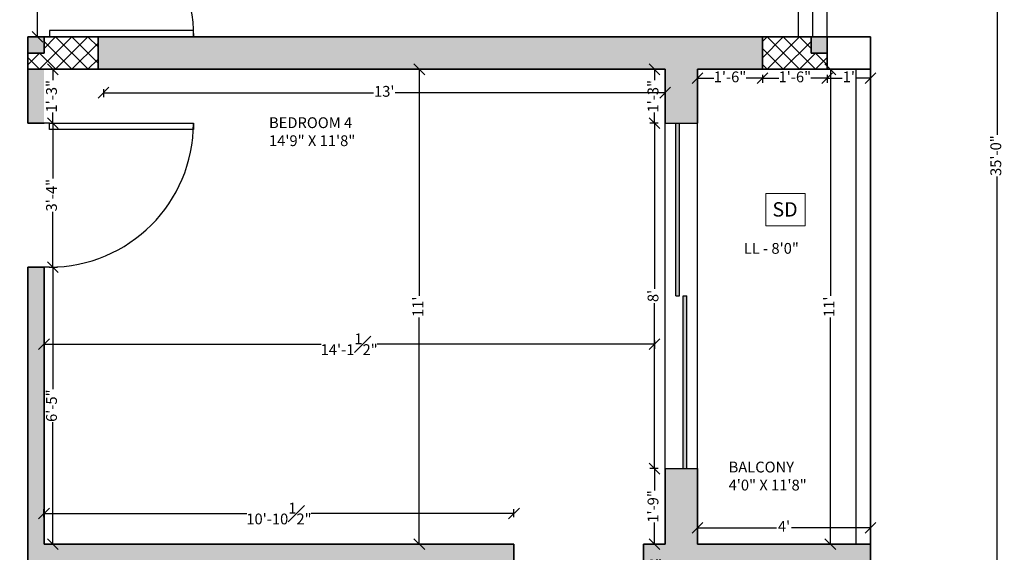
# Model space of a CAD drawing. Units: inches. Extents: x 1365 to 2091, y 1589 to 2091.
# Tile 7 of 8: x 1818 to 2091, y 1743 to 1891. Entities that reach past the tile are written whole.
import ezdxf

# ---------------------------------------------------------------- set-up
doc = ezdxf.new("R2010")
doc.units = ezdxf.units.IN
for name, color, linetype, lineweight in [('A-ANNO-DIMS', 2, 'Continuous', 18), ('A-ANNO-SYMB', 12, 'Continuous', 18), ('A-AREA-IDEN', 7, 'Continuous', 18), ('A-COLS', 7, 'Continuous', 35), ('A-COLS-MARK-PATT', 114, 'Continuous', 13), ('A-COLS-PATT', 1, 'Continuous', 13), ('A-DOOR', 4, 'Continuous', 25), ('A-DOOR-PATT', 143, 'Continuous', 13), ('A-FLOR-HRAL', 7, 'Continuous', 25), ('A-WALL', 7, 'Continuous', 35), ('A-WALL-PATT', 253, 'Continuous', 13)]:
    doc.layers.add(name, color=color, linetype=linetype, lineweight=lineweight)
doc.styles.get("Standard").update_dxf_attribs({"font": 'arial.ttf'})
doc.dimstyles.new('ISO-25', dxfattribs={"dimtxt": 3, "dimasz": 3, "dimexe": 1.25, "dimexo": 0.625, "dimtad": 0, "dimlunit": 4, "dimtxsty": 'Standard', "dimblk": 'OBLIQUE', "dimcen": 2.5, "dimclrd": 254, "dimclre": 254, "dimclrt": 1, "dimadec": 0, "dimazin": 0, "dimtfac": 1, "dimtmove": 0, "dimatfit": 3, "dimfxl": 1, "dimfxlon": 1, "dimfrac": 1, "dimarcsym": 0})

# ---------------------------------------------------------------- blocks, each defined once
blk = doc.blocks.new('*U5')
for p, q in [((0, 0), (0, -6)), ((40, 0), (40, -6))]:
    blk.add_line(p, q)
blk.add_lwpolyline([(0, 0), (0, 40), (1.75, 40), (1.75, 0)], close=True)
blk.add_arc((0, 0), 40, 0, 90)
blk = doc.blocks.new('_Oblique')
at = {"color": 0, "linetype": 'ByBlock', "lineweight": -2}
blk.add_line((-0.5, -0.5), (0.5, 0.5), dxfattribs=at)
blk = doc.blocks.new('*D61')
at = {"layer": 'A-ANNO-DIMS', "color": 0, "lineweight": -2, "transparency": 16777216}
for p, q in [((1929.47, 1876.86), (1927.22, 1876.86)), ((1928.47, 1876.86), (1928.47, 1813.89)), ((1928.47, 1744.86), (1928.47, 1807.83)), ((1929.47, 1744.86), (1927.22, 1744.86))]:
    blk.add_line(p, q, dxfattribs=at)
at = {"layer": 'Defpoints', "color": 0, "transparency": 16777216}
for p in [(1939.4, 1876.86), (1928.47, 1744.86), (1939.4, 1744.86)]:
    blk.add_point(p, dxfattribs=at)
at = {"layer": 'A-ANNO-DIMS', "color": 0, "lineweight": -2, "transparency": 16777216, "xscale": 3, "yscale": 3, "zscale": 3}
for p, rotation in [((1928.47, 1876.86), 90), ((1928.47, 1744.86), 270)]:
    blk.add_blockref('_Oblique', p, dxfattribs=dict(at, rotation=rotation))
at = {"layer": 'A-ANNO-DIMS', "color": 0, "transparency": 16777216, "insert": (1928.47, 1810.86), "char_height": 3, "attachment_point": 5, "rotation": 90}
blk.add_mtext("11'", dxfattribs=at)
blk = doc.blocks.new('*D62')
at = {"layer": 'A-ANNO-DIMS', "color": 0, "lineweight": -2, "transparency": 16777216}
for p, q in [((1825.72, 1876.86), (1827.97, 1876.86)), ((1826.72, 1876.86), (1826.72, 1873.83)), ((1826.72, 1861.86), (1826.72, 1864.89)), ((1825.72, 1861.86), (1827.97, 1861.86))]:
    blk.add_line(p, q, dxfattribs=at)
at = {"layer": 'Defpoints', "color": 0, "transparency": 16777216}
for p in [(1824.34, 1876.86), (1824.25, 1861.86), (1826.72, 1861.86)]:
    blk.add_point(p, dxfattribs=at)
at = {"layer": 'A-ANNO-DIMS', "color": 0, "lineweight": -2, "transparency": 16777216, "xscale": 3, "yscale": 3, "zscale": 3}
for p, rotation in [((1826.72, 1876.86), 90), ((1826.72, 1861.86), 270)]:
    blk.add_blockref('_Oblique', p, dxfattribs=dict(at, rotation=rotation))
at = {"layer": 'A-ANNO-DIMS', "color": 0, "transparency": 16777216, "insert": (1826.72, 1869.36), "char_height": 3, "attachment_point": 5, "rotation": 90}
blk.add_mtext('1\'-3"', dxfattribs=at)
blk = doc.blocks.new('*D63')
at = {"layer": 'A-ANNO-DIMS', "color": 0, "lineweight": -2, "transparency": 16777216}
for p, q in [((1825.72, 1861.86), (1827.97, 1861.86)), ((1826.72, 1861.86), (1826.72, 1846.47)), ((1826.72, 1821.86), (1826.72, 1837.25)), ((1825.72, 1821.86), (1827.97, 1821.86))]:
    blk.add_line(p, q, dxfattribs=at)
at = {"layer": 'Defpoints', "color": 0, "transparency": 16777216}
for p in [(1824.25, 1861.86), (1819.75, 1821.86), (1826.72, 1821.86)]:
    blk.add_point(p, dxfattribs=at)
at = {"layer": 'A-ANNO-DIMS', "color": 0, "lineweight": -2, "transparency": 16777216, "xscale": 3, "yscale": 3, "zscale": 3}
for p, rotation in [((1826.72, 1861.86), 90), ((1826.72, 1821.86), 270)]:
    blk.add_blockref('_Oblique', p, dxfattribs=dict(at, rotation=rotation))
at = {"layer": 'A-ANNO-DIMS', "color": 0, "transparency": 16777216, "insert": (1826.72, 1841.86), "char_height": 3, "attachment_point": 5, "rotation": 90}
blk.add_mtext('3\'-4"', dxfattribs=at)
blk = doc.blocks.new('*D64')
at = {"layer": 'A-ANNO-DIMS', "color": 0, "lineweight": -2, "transparency": 16777216}
for p, q in [((1825.72, 1821.86), (1827.97, 1821.86)), ((1826.72, 1821.86), (1826.72, 1787.98)), ((1826.72, 1744.86), (1826.72, 1778.74)), ((1825.72, 1744.86), (1827.97, 1744.86))]:
    blk.add_line(p, q, dxfattribs=at)
at = {"layer": 'Defpoints', "color": 0, "transparency": 16777216}
for p in [(1819.75, 1821.86), (1824.25, 1744.86), (1826.72, 1744.86)]:
    blk.add_point(p, dxfattribs=at)
at = {"layer": 'A-ANNO-DIMS', "color": 0, "lineweight": -2, "transparency": 16777216, "xscale": 3, "yscale": 3, "zscale": 3}
for p, rotation in [((1826.72, 1821.86), 90), ((1826.72, 1744.86), 270)]:
    blk.add_blockref('_Oblique', p, dxfattribs=dict(at, rotation=rotation))
at = {"layer": 'A-ANNO-DIMS', "color": 0, "transparency": 16777216, "insert": (1826.72, 1783.36), "char_height": 3, "attachment_point": 5, "rotation": 90}
blk.add_mtext('6\'-5"', dxfattribs=at)
blk = doc.blocks.new('*D65')
at = {"layer": 'A-ANNO-DIMS', "color": 0, "lineweight": -2, "transparency": 16777216}
for p, q in [((1824.25, 1752.38), (1824.25, 1754.63)), ((1824.25, 1753.38), (1880.56, 1753.38)), ((1954.75, 1753.38), (1898.45, 1753.38)), ((1954.75, 1752.38), (1954.75, 1754.63))]:
    blk.add_line(p, q, dxfattribs=at)
at = {"layer": 'Defpoints', "color": 0, "transparency": 16777216}
for p in [(1954.75, 1753.38), (1824.25, 1744.86), (1954.75, 1744.86)]:
    blk.add_point(p, dxfattribs=at)
at = {"layer": 'A-ANNO-DIMS', "color": 0, "lineweight": -2, "transparency": 16777216, "xscale": 3, "yscale": 3, "zscale": 3, "rotation": 180}
blk.add_blockref('_Oblique', (1824.25, 1753.38), dxfattribs=at)
at = {"layer": 'A-ANNO-DIMS', "color": 0, "lineweight": -2, "transparency": 16777216, "xscale": 3, "yscale": 3, "zscale": 3}
blk.add_blockref('_Oblique', (1954.75, 1753.38), dxfattribs=at)
at = {"layer": 'A-ANNO-DIMS', "color": 0, "transparency": 16777216, "insert": (1889.5, 1753.38), "char_height": 3, "attachment_point": 5}
blk.add_mtext('10\'-10{\\H1x;\\S1#2;}"', dxfattribs=at)
blk = doc.blocks.new('*D66')
at = {"layer": 'A-ANNO-DIMS', "color": 0, "lineweight": -2, "transparency": 16777216}
for p, q in [((1840.75, 1871.34), (1840.75, 1869.09)), ((1840.75, 1870.34), (1915.72, 1870.34)), ((1996.75, 1870.34), (1921.78, 1870.34)), ((1996.75, 1871.34), (1996.75, 1869.09))]:
    blk.add_line(p, q, dxfattribs=at)
at = {"layer": 'Defpoints', "color": 0, "transparency": 16777216}
for p in [(1840.75, 1876.86), (1996.75, 1876.86), (1840.75, 1870.34)]:
    blk.add_point(p, dxfattribs=at)
at = {"layer": 'A-ANNO-DIMS', "color": 0, "lineweight": -2, "transparency": 16777216, "xscale": 3, "yscale": 3, "zscale": 3, "rotation": 180}
blk.add_blockref('_Oblique', (1840.75, 1870.34), dxfattribs=at)
at = {"layer": 'A-ANNO-DIMS', "color": 0, "lineweight": -2, "transparency": 16777216, "xscale": 3, "yscale": 3, "zscale": 3}
blk.add_blockref('_Oblique', (1996.75, 1870.34), dxfattribs=at)
at = {"layer": 'A-ANNO-DIMS', "color": 0, "transparency": 16777216, "insert": (1918.75, 1870.34), "char_height": 3, "attachment_point": 5}
blk.add_mtext("13'", dxfattribs=at)
blk = doc.blocks.new('*D67')
at = {"layer": 'A-ANNO-DIMS', "color": 0, "lineweight": -2, "transparency": 16777216}
for p, q in [((1994.76, 1765.86), (1992.51, 1765.86)), ((1993.76, 1765.86), (1993.76, 1759.83)), ((1993.76, 1744.86), (1993.76, 1750.89)), ((1994.76, 1744.86), (1992.51, 1744.86))]:
    blk.add_line(p, q, dxfattribs=at)
at = {"layer": 'Defpoints', "color": 0, "transparency": 16777216}
for p in [(1993.76, 1765.86), (1996.75, 1765.86), (1996.75, 1744.86)]:
    blk.add_point(p, dxfattribs=at)
at = {"layer": 'A-ANNO-DIMS', "color": 0, "lineweight": -2, "transparency": 16777216, "xscale": 3, "yscale": 3, "zscale": 3}
for p, rotation in [((1993.76, 1765.86), 90), ((1993.76, 1744.86), 270)]:
    blk.add_blockref('_Oblique', p, dxfattribs=dict(at, rotation=rotation))
at = {"layer": 'A-ANNO-DIMS', "color": 0, "transparency": 16777216, "insert": (1993.76, 1755.36), "char_height": 3, "attachment_point": 5, "rotation": 90}
blk.add_mtext('1\'-9"', dxfattribs=at)
blk = doc.blocks.new('*D68')
at = {"layer": 'A-ANNO-DIMS', "color": 0, "lineweight": -2, "transparency": 16777216}
for p, q in [((1990.75, 1739.68), (1990.75, 1737.43)), ((1996.75, 1739.68), (1996.75, 1737.43)), ((1990.75, 1738.68), (1991.4, 1738.68)), ((1996.75, 1738.68), (1996.11, 1738.68))]:
    blk.add_line(p, q, dxfattribs=at)
at = {"layer": 'Defpoints', "color": 0, "transparency": 16777216}
for p in [(1990.75, 1744.86), (1996.75, 1744.86), (1996.75, 1738.68)]:
    blk.add_point(p, dxfattribs=at)
at = {"layer": 'A-ANNO-DIMS', "color": 0, "lineweight": -2, "transparency": 16777216, "xscale": 3, "yscale": 3, "zscale": 3, "rotation": 180}
blk.add_blockref('_Oblique', (1990.75, 1738.68), dxfattribs=at)
at = {"layer": 'A-ANNO-DIMS', "color": 0, "lineweight": -2, "transparency": 16777216, "xscale": 3, "yscale": 3, "zscale": 3}
blk.add_blockref('_Oblique', (1996.75, 1738.68), dxfattribs=at)
at = {"layer": 'A-ANNO-DIMS', "color": 0, "transparency": 16777216, "insert": (1993.75, 1738.68), "char_height": 3, "attachment_point": 5}
blk.add_mtext('6"', dxfattribs=at)
blk = doc.blocks.new('*D69')
at = {"layer": 'A-ANNO-DIMS', "color": 0, "lineweight": -2, "transparency": 16777216}
for p, q in [((1994.76, 1861.86), (1992.51, 1861.86)), ((1993.76, 1861.86), (1993.76, 1815.86)), ((1993.76, 1765.86), (1993.76, 1811.85)), ((1994.76, 1765.86), (1992.51, 1765.86))]:
    blk.add_line(p, q, dxfattribs=at)
at = {"layer": 'Defpoints', "color": 0, "transparency": 16777216}
for p in [(1993.76, 1861.86), (1996.75, 1861.86), (1996.75, 1765.86)]:
    blk.add_point(p, dxfattribs=at)
at = {"layer": 'A-ANNO-DIMS', "color": 0, "lineweight": -2, "transparency": 16777216, "xscale": 3, "yscale": 3, "zscale": 3}
for p, rotation in [((1993.76, 1861.86), 90), ((1993.76, 1765.86), 270)]:
    blk.add_blockref('_Oblique', p, dxfattribs=dict(at, rotation=rotation))
at = {"layer": 'A-ANNO-DIMS', "color": 0, "transparency": 16777216, "insert": (1993.76, 1813.86), "char_height": 3, "attachment_point": 5, "rotation": 90}
blk.add_mtext("8'", dxfattribs=at)
blk = doc.blocks.new('*D70')
at = {"layer": 'A-ANNO-DIMS', "color": 0, "lineweight": -2, "transparency": 16777216}
for p, q in [((1994.76, 1876.86), (1992.51, 1876.86)), ((1993.76, 1876.86), (1993.76, 1873.83)), ((1993.76, 1861.86), (1993.76, 1864.89)), ((1994.76, 1861.86), (1992.51, 1861.86))]:
    blk.add_line(p, q, dxfattribs=at)
at = {"layer": 'Defpoints', "color": 0, "transparency": 16777216}
for p in [(1993.76, 1876.86), (1996.75, 1876.86), (1996.75, 1861.86)]:
    blk.add_point(p, dxfattribs=at)
at = {"layer": 'A-ANNO-DIMS', "color": 0, "lineweight": -2, "transparency": 16777216, "xscale": 3, "yscale": 3, "zscale": 3}
for p, rotation in [((1993.76, 1876.86), 90), ((1993.76, 1861.86), 270)]:
    blk.add_blockref('_Oblique', p, dxfattribs=dict(at, rotation=rotation))
at = {"layer": 'A-ANNO-DIMS', "color": 0, "transparency": 16777216, "insert": (1993.76, 1869.36), "char_height": 3, "attachment_point": 5, "rotation": 90}
blk.add_mtext('1\'-3"', dxfattribs=at)
blk = doc.blocks.new('*D71')
at = {"layer": 'A-ANNO-DIMS', "color": 0, "lineweight": -2, "transparency": 16777216}
for p, q in [((2005.75, 1875.36), (2005.75, 1873.11)), ((2005.75, 1874.36), (2010.28, 1874.36)), ((2023.75, 1874.36), (2019.22, 1874.36)), ((2023.75, 1875.36), (2023.75, 1873.11))]:
    blk.add_line(p, q, dxfattribs=at)
at = {"layer": 'Defpoints', "color": 0, "transparency": 16777216}
for p in [(2005.75, 1876.86), (2023.75, 1876.86), (2023.75, 1874.36)]:
    blk.add_point(p, dxfattribs=at)
at = {"layer": 'A-ANNO-DIMS', "color": 0, "lineweight": -2, "transparency": 16777216, "xscale": 3, "yscale": 3, "zscale": 3, "rotation": 180}
blk.add_blockref('_Oblique', (2005.75, 1874.36), dxfattribs=at)
at = {"layer": 'A-ANNO-DIMS', "color": 0, "lineweight": -2, "transparency": 16777216, "xscale": 3, "yscale": 3, "zscale": 3}
blk.add_blockref('_Oblique', (2023.75, 1874.36), dxfattribs=at)
at = {"layer": 'A-ANNO-DIMS', "color": 0, "transparency": 16777216, "insert": (2014.75, 1874.36), "char_height": 3, "attachment_point": 5}
blk.add_mtext('1\'-6"', dxfattribs=at)
blk = doc.blocks.new('*D72')
at = {"layer": 'A-ANNO-DIMS', "color": 0, "lineweight": -2, "transparency": 16777216}
for p, q in [((2023.75, 1875.36), (2023.75, 1873.11)), ((2023.75, 1874.36), (2028.28, 1874.36)), ((2041.75, 1874.36), (2037.22, 1874.36)), ((2041.75, 1875.36), (2041.75, 1873.11))]:
    blk.add_line(p, q, dxfattribs=at)
at = {"layer": 'Defpoints', "color": 0, "transparency": 16777216}
for p in [(2023.75, 1876.86), (2041.75, 1876.86), (2041.75, 1874.36)]:
    blk.add_point(p, dxfattribs=at)
at = {"layer": 'A-ANNO-DIMS', "color": 0, "lineweight": -2, "transparency": 16777216, "xscale": 3, "yscale": 3, "zscale": 3, "rotation": 180}
blk.add_blockref('_Oblique', (2023.75, 1874.36), dxfattribs=at)
at = {"layer": 'A-ANNO-DIMS', "color": 0, "lineweight": -2, "transparency": 16777216, "xscale": 3, "yscale": 3, "zscale": 3}
blk.add_blockref('_Oblique', (2041.75, 1874.36), dxfattribs=at)
at = {"layer": 'A-ANNO-DIMS', "color": 0, "transparency": 16777216, "insert": (2032.75, 1874.36), "char_height": 3, "attachment_point": 5}
blk.add_mtext('1\'-6"', dxfattribs=at)
blk = doc.blocks.new('*D73')
at = {"layer": 'A-ANNO-DIMS', "color": 0, "lineweight": -2, "transparency": 16777216}
for p, q in [((2041.75, 1875.36), (2041.75, 1873.11)), ((2041.75, 1874.36), (2045.89, 1874.36)), ((2053.75, 1874.36), (2049.62, 1874.36)), ((2053.75, 1875.36), (2053.75, 1873.11))]:
    blk.add_line(p, q, dxfattribs=at)
at = {"layer": 'Defpoints', "color": 0, "transparency": 16777216}
for p in [(2041.75, 1876.86), (2053.75, 1876.86), (2053.75, 1874.36)]:
    blk.add_point(p, dxfattribs=at)
at = {"layer": 'A-ANNO-DIMS', "color": 0, "lineweight": -2, "transparency": 16777216, "xscale": 3, "yscale": 3, "zscale": 3, "rotation": 180}
blk.add_blockref('_Oblique', (2041.75, 1874.36), dxfattribs=at)
at = {"layer": 'A-ANNO-DIMS', "color": 0, "lineweight": -2, "transparency": 16777216, "xscale": 3, "yscale": 3, "zscale": 3}
blk.add_blockref('_Oblique', (2053.75, 1874.36), dxfattribs=at)
at = {"layer": 'A-ANNO-DIMS', "color": 0, "transparency": 16777216, "insert": (2047.75, 1874.36), "char_height": 3, "attachment_point": 5}
blk.add_mtext("1'", dxfattribs=at)
blk = doc.blocks.new('*D74')
at = {"layer": 'A-ANNO-DIMS', "color": 0, "lineweight": -2, "transparency": 16777216}
for p, q in [((2043.63, 1876.86), (2041.38, 1876.86)), ((2042.63, 1876.86), (2042.63, 1813.89)), ((2042.63, 1744.86), (2042.63, 1807.83)), ((2043.63, 1744.86), (2041.38, 1744.86))]:
    blk.add_line(p, q, dxfattribs=at)
at = {"layer": 'Defpoints', "color": 0, "transparency": 16777216}
for p in [(2053.75, 1876.86), (2042.63, 1744.86), (2053.75, 1744.86)]:
    blk.add_point(p, dxfattribs=at)
at = {"layer": 'A-ANNO-DIMS', "color": 0, "lineweight": -2, "transparency": 16777216, "xscale": 3, "yscale": 3, "zscale": 3}
for p, rotation in [((2042.63, 1876.86), 90), ((2042.63, 1744.86), 270)]:
    blk.add_blockref('_Oblique', p, dxfattribs=dict(at, rotation=rotation))
at = {"layer": 'A-ANNO-DIMS', "color": 0, "transparency": 16777216, "insert": (2042.63, 1810.86), "char_height": 3, "attachment_point": 5, "rotation": 90}
blk.add_mtext("11'", dxfattribs=at)
blk = doc.blocks.new('*D75')
at = {"layer": 'A-ANNO-DIMS', "color": 0, "lineweight": -2, "transparency": 16777216}
for p, q in [((2005.75, 1748.43), (2005.75, 1750.68)), ((2053.75, 1748.43), (2053.75, 1750.68)), ((2005.75, 1749.43), (2027.69, 1749.43)), ((2053.75, 1749.43), (2031.82, 1749.43))]:
    blk.add_line(p, q, dxfattribs=at)
at = {"layer": 'Defpoints', "color": 0, "transparency": 16777216}
for p in [(2053.75, 1749.43), (2005.75, 1744.86), (2053.75, 1744.86)]:
    blk.add_point(p, dxfattribs=at)
at = {"layer": 'A-ANNO-DIMS', "color": 0, "lineweight": -2, "transparency": 16777216, "xscale": 3, "yscale": 3, "zscale": 3, "rotation": 180}
blk.add_blockref('_Oblique', (2005.75, 1749.43), dxfattribs=at)
at = {"layer": 'A-ANNO-DIMS', "color": 0, "lineweight": -2, "transparency": 16777216, "xscale": 3, "yscale": 3, "zscale": 3}
blk.add_blockref('_Oblique', (2053.75, 1749.43), dxfattribs=at)
at = {"layer": 'A-ANNO-DIMS', "color": 0, "transparency": 16777216, "insert": (2029.75, 1749.43), "char_height": 3, "attachment_point": 5}
blk.add_mtext("4'", dxfattribs=at)
blk = doc.blocks.new('*D86')
at = {"layer": 'A-ANNO-DIMS', "color": 0, "lineweight": -2, "transparency": 16777216}
for p, q in [((1824.25, 1801.44), (1824.25, 1799.19)), ((1824.25, 1800.44), (1901.22, 1800.44)), ((1993.76, 1800.44), (1916.79, 1800.44)), ((1993.76, 1801.44), (1993.76, 1799.19))]:
    blk.add_line(p, q, dxfattribs=at)
at = {"layer": 'Defpoints', "color": 0, "transparency": 16777216}
for p in [(1824.25, 1821.86), (1993.76, 1821.86), (1993.76, 1800.44)]:
    blk.add_point(p, dxfattribs=at)
at = {"layer": 'A-ANNO-DIMS', "color": 0, "lineweight": -2, "transparency": 16777216, "xscale": 3, "yscale": 3, "zscale": 3, "rotation": 180}
blk.add_blockref('_Oblique', (1824.25, 1800.44), dxfattribs=at)
at = {"layer": 'A-ANNO-DIMS', "color": 0, "lineweight": -2, "transparency": 16777216, "xscale": 3, "yscale": 3, "zscale": 3}
blk.add_blockref('_Oblique', (1993.76, 1800.44), dxfattribs=at)
at = {"layer": 'A-ANNO-DIMS', "color": 0, "transparency": 16777216, "insert": (1909, 1800.44), "char_height": 3, "attachment_point": 5}
blk.add_mtext('14\'-1{\\H1x;\\S1#2;}"', dxfattribs=at)
blk = doc.blocks.new('*D92')
at = {"layer": 'A-ANNO-DIMS', "color": 0, "lineweight": -2, "transparency": 16777216}
for p, q in [((1821.45, 1925.83), (1823.7, 1925.83)), ((1822.45, 1925.83), (1822.45, 1910.45)), ((1822.45, 1885.86), (1822.45, 1901.23)), ((1821.45, 1885.86), (1823.7, 1885.86))]:
    blk.add_line(p, q, dxfattribs=at)
at = {"layer": 'Defpoints', "color": 0, "transparency": 16777216}
for p in [(1819.75, 1925.83), (1819.75, 1885.86), (1822.45, 1885.86)]:
    blk.add_point(p, dxfattribs=at)
at = {"layer": 'A-ANNO-DIMS', "color": 0, "lineweight": -2, "transparency": 16777216, "xscale": 3, "yscale": 3, "zscale": 3}
for p, rotation in [((1822.45, 1925.83), 90), ((1822.45, 1885.86), 270)]:
    blk.add_blockref('_Oblique', p, dxfattribs=dict(at, rotation=rotation))
at = {"layer": 'A-ANNO-DIMS', "color": 0, "transparency": 16777216, "insert": (1822.45, 1905.84), "char_height": 3, "attachment_point": 5, "rotation": 90}
blk.add_mtext('3\'-4"', dxfattribs=at)
blk = doc.blocks.new('*D123')
at = {"layer": 'A-ANNO-DIMS', "color": 254, "lineweight": -2, "transparency": 16777216}
for p, q in [((2087.95, 2062.86), (2090.2, 2062.86)), ((2088.95, 2062.86), (2088.95, 1858.63)), ((2088.95, 1642.86), (2088.95, 1847.08)), ((2087.95, 1642.86), (2090.2, 1642.86))]:
    blk.add_line(p, q, dxfattribs=at)
at = {"layer": 'Defpoints', "color": 0, "transparency": 16777216}
for p in [(2053.75, 2062.86), (2088.95, 2062.86), (2053.75, 1642.86)]:
    blk.add_point(p, dxfattribs=at)
at = {"layer": 'A-ANNO-DIMS', "color": 254, "lineweight": -2, "transparency": 16777216, "xscale": 3, "yscale": 3, "zscale": 3}
for p, rotation in [((2088.95, 2062.86), 90), ((2088.95, 1642.86), 270)]:
    blk.add_blockref('_Oblique', p, dxfattribs=dict(at, rotation=rotation))
at = {"layer": 'A-ANNO-DIMS', "color": 1, "transparency": 16777216, "insert": (2088.95, 1852.86), "char_height": 3, "attachment_point": 5, "rotation": 90}
blk.add_mtext('35\'-0"', dxfattribs=at)

msp = doc.modelspace()

# ---------------------------------------------------------------- hatches: boundary and pattern name
at = {"layer": 'A-COLS-MARK-PATT'}
h = msp.add_hatch(color=256, dxfattribs=at)
h.dxf.hatch_style = 1
h.paths.add_polyline_path([(1398.254, 2062.858), (1393.754, 2062.858), (1393.754, 2058.358), (1398.254, 2058.358)])
h.paths.add_polyline_path([(1398.254, 1872.358), (1393.754, 1872.358), (1393.754, 1867.858), (1398.254, 1867.858)])
h.paths.add_polyline_path([(1398.254, 1807.858), (1393.754, 1807.858), (1393.754, 1803.358), (1398.254, 1803.358)])
h.paths.add_polyline_path([(1398.254, 1647.358), (1393.754, 1647.358), (1393.754, 1642.858), (1398.254, 1642.858)])
h.paths.add_polyline_path([(1638.254, 1647.358), (1633.754, 1647.358), (1633.754, 1642.858), (1638.254, 1642.858)])
h.paths.add_polyline_path([(1638.254, 1732.858), (1633.754, 1732.858), (1633.754, 1728.358), (1638.254, 1728.358)])
h.paths.add_polyline_path([(1647.254, 1876.858), (1642.754, 1876.858), (1642.754, 1872.358), (1647.254, 1872.358)])
h.paths.add_polyline_path([(1647.254, 1803.358), (1642.754, 1803.358), (1642.754, 1798.858), (1647.254, 1798.858)])
h.paths.add_polyline_path([(1647.254, 2062.858), (1642.754, 2062.858), (1642.754, 2058.358), (1647.254, 2058.358)])
h.paths.add_polyline_path([(1824.254, 2062.858), (1819.754, 2062.858), (1819.754, 2058.358), (1824.254, 2058.358)])
h.paths.add_polyline_path([(1824.254, 1885.858), (1819.754, 1885.858), (1819.754, 1881.358), (1824.254, 1881.358)])
h.paths.add_polyline_path([(1828.754, 1647.358), (1824.254, 1647.358), (1824.254, 1642.858), (1828.754, 1642.858)])
h.paths.add_polyline_path([(1948.754, 1647.358), (1944.254, 1647.358), (1944.254, 1642.858), (1948.754, 1642.858)])
h.paths.add_polyline_path([(2041.754, 1647.358), (2037.254, 1647.358), (2037.254, 1642.858), (2041.754, 1642.858)])
h.paths.add_polyline_path([(2041.754, 1885.858), (2037.254, 1885.858), (2037.254, 1881.358), (2041.754, 1881.358)])
h.paths.add_polyline_path([(2041.754, 2062.858), (2037.254, 2062.858), (2037.254, 2058.358), (2041.754, 2058.358)])
at = {"layer": 'A-COLS-PATT'}
h = msp.add_hatch(dxfattribs=at)
h.set_pattern_fill('ANSI37', color=256)
h.paths.add_polyline_path([(1642.754, 1803.358), (1647.254, 1803.358), (1647.254, 1807.858), (1629.254, 1807.858), (1629.254, 1798.858), (1633.754, 1798.858), (1642.754, 1798.858)])
h.paths.add_polyline_path([(1647.254, 1872.358), (1642.754, 1872.358), (1642.754, 1876.858), (1641.254, 1876.858), (1623.254, 1876.858), (1623.254, 1867.858), (1638.254, 1867.858), (1647.254, 1867.858)])
h.paths.add_polyline_path([(1647.254, 2058.358), (1642.754, 2058.358), (1642.754, 2062.858), (1638.254, 2062.858), (1638.254, 2053.858), (1647.254, 2053.858)])
h.paths.add_polyline_path([(1642.754, 2053.858), (1638.254, 2053.858), (1638.254, 2041.858), (1642.754, 2041.858)])
h.paths.add_polyline_path([(1647.254, 2053.858), (1642.754, 2053.858), (1642.754, 2041.858), (1647.254, 2041.858)])
h.paths.add_polyline_path([(1828.754, 2062.858), (1824.254, 2062.858), (1824.254, 2058.358), (1819.754, 2058.358), (1819.754, 2038.858), (1828.754, 2038.858)])
h.paths.add_polyline_path([(1839.254, 1885.858), (1825.754, 1885.858), (1824.254, 1885.858), (1824.254, 1881.358), (1819.754, 1881.358), (1819.754, 1876.858), (1839.254, 1876.858)])
h.paths.add_polyline_path([(2041.754, 1881.358), (2037.254, 1881.358), (2037.254, 1885.858), (2023.754, 1885.858), (2023.754, 1876.858), (2041.754, 1876.858)])
h.paths.add_polyline_path([(1828.754, 1666.858), (1819.754, 1666.858), (1819.754, 1642.858), (1824.254, 1642.858), (1824.254, 1647.358), (1828.754, 1647.358)])
h.paths.add_polyline_path([(1944.254, 1647.358), (1948.754, 1647.358), (1948.754, 1651.858), (1930.754, 1651.858), (1930.754, 1642.858), (1944.254, 1642.858)])
h.paths.add_polyline_path([(2037.254, 1647.358), (2041.754, 1647.358), (2041.754, 1651.858), (2023.754, 1651.858), (2023.754, 1642.858), (2037.254, 1642.858)])
at = {"layer": 'A-DOOR-PATT'}
h = msp.add_hatch(color=256, dxfattribs=at)
h.dxf.hatch_style = 1
h.paths.add_polyline_path([(2000.754, 1861.858), (1999.754, 1861.858), (1999.754, 1813.858), (2000.754, 1813.858)])
h.paths.add_polyline_path([(2002.754, 1813.858), (2001.754, 1813.858), (2001.754, 1765.858), (2002.754, 1765.858)])
at = {"layer": 'A-WALL-PATT'}
h = msp.add_hatch(color=256, dxfattribs=at)
h.dxf.hatch_style = 1
h.paths.add_polyline_path([(1996.754, 1876.858), (1996.754, 1861.858), (2005.754, 1861.858), (2005.754, 1876.858), (2023.754, 1876.858), (2023.754, 1885.858), (1839.254, 1885.858), (1839.254, 1876.858)])
h.paths.add_polyline_path([(2053.754, 1744.858), (2005.754, 1744.858), (2005.754, 1765.858), (1996.754, 1765.858), (1996.754, 1744.858), (1990.754, 1744.858), (1990.754, 1740.358), (2044.754, 1740.358), (2044.754, 1651.858), (2044.754, 1642.858), (2053.754, 1642.858)])
h = msp.add_hatch(color=256, dxfattribs=at)
h.dxf.hatch_style = 1
h.paths.add_polyline_path([(1824.254, 1876.858), (1819.754, 1876.858), (1819.754, 1861.858), (1824.254, 1861.858)])
h = msp.add_hatch(color=256, dxfattribs=at)
h.dxf.hatch_style = 1
h.paths.add_polyline_path([(1402.754, 1753.858), (1393.754, 1753.858), (1393.754, 1663.858), (1402.754, 1663.858)])
h.paths.add_polyline_path([(1533.254, 1804.358), (1476.254, 1804.358), (1476.254, 1816.358), (1471.754, 1816.358), (1471.754, 1804.358), (1402.754, 1804.358), (1402.754, 1799.858), (1533.254, 1799.858)])
h.paths.add_polyline_path([(1638.254, 1714.858), (1633.754, 1714.858), (1633.754, 1666.858), (1638.254, 1666.858)])
h.paths.add_polyline_path([(1638.254, 1740.858), (1633.754, 1740.858), (1633.754, 1732.858), (1638.254, 1732.858)])
h.paths.add_polyline_path([(1954.754, 1744.858), (1948.754, 1744.858), (1944.254, 1744.858), (1824.254, 1744.858), (1824.254, 1821.858), (1819.754, 1821.858), (1819.754, 1666.858), (1824.254, 1666.858), (1824.254, 1740.358), (1944.254, 1740.358), (1948.754, 1740.358), (1954.754, 1740.358)])
h.paths.add_polyline_path([(1948.754, 1698.358), (1944.254, 1698.358), (1944.254, 1651.858), (1948.754, 1651.858)])
h.paths.add_polyline_path([(1948.754, 1740.358), (1944.254, 1740.358), (1944.254, 1734.358), (1948.754, 1734.358)], flags=17)

# ---------------------------------------------------------------- linework, layer by layer
at = {"layer": 'A-ANNO-SYMB'}
msp.add_lwpolyline([(2024.688, 1842.367), (2035.577, 1842.367), (2035.577, 1833.329), (2024.688, 1833.329)], close=True, dxfattribs=at)
at = {"layer": 'A-COLS'}
for p, q in [((1824.254, 1885.858), (1824.254, 1881.358)), ((1839.254, 1885.858), (1839.254, 1876.858)), ((2023.754, 1876.858), (2023.754, 1885.858)), ((2037.254, 1881.358), (2037.254, 1885.858)), ((2041.754, 1885.858), (2041.754, 1876.858)), ((2041.754, 1885.858), (2041.754, 1881.358)), ((1824.254, 1881.358), (1819.754, 1881.358)), ((2041.754, 1881.358), (2037.254, 1881.358)), ((2041.754, 1876.858), (2023.754, 1876.858))]:
    msp.add_line(p, q, dxfattribs=at)
at = {"layer": 'A-DOOR'}
for p, q in [((1996.754, 1765.858), (1996.754, 1861.858)), ((1996.754, 1861.858), (2005.754, 1861.858)), ((1999.754, 1813.858), (1999.754, 1861.858)), ((2000.754, 1813.858), (2000.754, 1861.858)), ((2005.754, 1765.858), (2005.754, 1861.858)), ((1999.754, 1813.858), (2000.754, 1813.858)), ((2001.754, 1765.858), (2001.754, 1813.858)), ((2001.754, 1813.858), (2002.754, 1813.858)), ((2002.754, 1765.858), (2002.754, 1813.858)), ((1996.754, 1765.858), (2005.754, 1765.858))]:
    msp.add_line(p, q, dxfattribs=at)
at = {"layer": 'A-FLOR-HRAL'}
for p, q in [((2033.754, 1885.858), (2033.754, 1966.858)), ((2037.754, 1885.858), (2037.754, 1966.858)), ((2041.754, 1885.858), (2041.754, 1966.858)), ((2049.754, 1744.858), (2049.754, 1876.858))]:
    msp.add_line(p, q, dxfattribs=at)
at = {"layer": 'A-WALL'}
for p, q in [((2053.754, 1885.858), (1819.754, 1885.858)), ((1819.754, 1885.858), (1819.754, 1861.858)), ((1840.754, 1885.858), (1836.254, 1885.858)), ((2053.754, 1885.858), (2053.754, 1642.858)), ((1819.754, 1876.858), (1996.754, 1876.858)), ((1996.754, 1861.858), (1996.754, 1876.858)), ((2005.754, 1861.858), (2005.754, 1876.858)), ((2005.754, 1876.858), (2053.754, 1876.858)), ((1819.754, 1861.858), (1824.254, 1861.858)), ((1824.254, 1821.858), (1819.754, 1821.858)), ((1819.754, 1821.858), (1819.754, 1666.858)), ((1824.254, 1744.858), (1824.254, 1821.858)), ((1996.754, 1744.858), (1996.754, 1765.858)), ((2005.754, 1744.858), (2005.754, 1765.858)), ((1944.254, 1744.858), (1824.254, 1744.858)), ((1948.754, 1744.858), (1944.254, 1744.858)), ((1954.754, 1744.858), (1948.754, 1744.858)), ((1954.754, 1744.858), (1954.754, 1740.358)), ((1990.754, 1740.358), (1990.754, 1744.858)), ((1990.754, 1744.858), (1996.754, 1744.858)), ((2005.754, 1744.858), (2053.754, 1744.858))]:
    msp.add_line(p, q, dxfattribs=at)

# ---------------------------------------------------------------- block references
at = {"layer": 'A-DOOR', "xscale": -1, "rotation": 270}
msp.add_blockref('*U5', (1825.754, 1885.858), dxfattribs=at)
at = {"layer": 'A-DOOR', "rotation": 270}
msp.add_blockref('*U5', (1825.754, 1861.858), dxfattribs=at)

# ---------------------------------------------------------------- texts
at = {"layer": 'A-ANNO-SYMB', "attachment_point": 1}
for s, width, insert, char_height in [('{SD}', 14.51356, (2026.528, 1839.916), 4), ('{LL - 8\'0"}', 24.3857, (2018.553, 1828.581), 3)]:
    msp.add_mtext_dynamic_manual_height_columns(s, width=width, gutter_width=12.5, heights=[0], dxfattribs=dict(at, insert=insert, char_height=char_height))
at = {"layer": 'A-AREA-IDEN', "char_height": 3, "attachment_point": 1}
for s, insert in [('{BEDROOM 4\\P14\'9" X 11\'8"}', (1886.732, 1863.507)), ('{BALCONY\\P4\'0" X 11\'8"}', (2014.359, 1767.805))]:
    msp.add_mtext_dynamic_manual_height_columns(s, width=33.58604, gutter_width=12.5, heights=[0], dxfattribs=dict(at, insert=insert))

# ---------------------------------------------------------------- dimensions: what is measured, and where the dimension line sits
at = {"layer": 'A-ANNO-DIMS'}
for base, p1, p2, override, picture, middle in [((2088.954, 2062.858), (2053.754, 1642.858), (2053.754, 2062.858), {"dimdec": 1, "dimlfac": 1, "dimrnd": 0, "dimzin": 1, "dimdsep": 46, "dimlunit": 4, "dimfrac": 2}, '*D123', (2088.954, 1852.858)), ((1822.447, 1885.858), (1819.754, 1925.829), (1819.754, 1885.858), {"dimclrd": 0, "dimclre": 0, "dimclrt": 0}, '*D92', (1822.447, 1905.843)), ((1826.723, 1861.858), (1824.344, 1876.858), (1824.254, 1861.858), {"dimclrd": 0, "dimclre": 0, "dimclrt": 0}, '*D62', (1826.723, 1869.358)), ((1928.468, 1744.858), (1939.403, 1876.858), (1939.403, 1744.858), {"dimclrd": 0, "dimclre": 0, "dimclrt": 0}, '*D61', (1928.468, 1810.858)), ((1993.755, 1876.858), (1996.754, 1861.858), (1996.754, 1876.858), {"dimclrd": 0, "dimclre": 0, "dimclrt": 0, "dimtmove": 1}, '*D70', (1993.755, 1869.358)), ((2042.63, 1744.858), (2053.754, 1876.858), (2053.754, 1744.858), {"dimclrd": 0, "dimclre": 0, "dimclrt": 0}, '*D74', (2042.63, 1810.858)), ((1826.723, 1821.858), (1824.254, 1861.858), (1819.754, 1821.858), {"dimclrd": 0, "dimclre": 0, "dimclrt": 0, "dimtmove": 1}, '*D63', (1826.723, 1841.858)), ((1993.755, 1861.858), (1996.754, 1765.858), (1996.754, 1861.858), {"dimclrd": 0, "dimclre": 0, "dimclrt": 0, "dimtmove": 1}, '*D69', (1993.755, 1813.858)), ((1826.723, 1744.858), (1819.754, 1821.858), (1824.254, 1744.858), {"dimclrd": 0, "dimclre": 0, "dimclrt": 0, "dimtmove": 1}, '*D64', (1826.723, 1783.358)), ((1993.755, 1765.858), (1996.754, 1744.858), (1996.754, 1765.858), {"dimclrd": 0, "dimclre": 0, "dimclrt": 0}, '*D67', (1993.755, 1755.358))]:
    dim = msp.add_linear_dim(base=base, p1=p1, p2=p2, angle=90, dimstyle='ISO-25', override=override, dxfattribs=at)
    dim.commit()
    dim.dimension.update_dxf_attribs({"geometry": picture, "text_midpoint": middle})
for base, p1, p2, override, picture, middle in [((1840.754, 1870.342), (1996.754, 1876.858), (1840.754, 1876.858), {"dimclrd": 0, "dimclre": 0, "dimclrt": 0}, '*D66', (1918.754, 1870.342)), ((2023.754, 1874.356), (2005.754, 1876.858), (2023.754, 1876.858), {"dimclrd": 0, "dimclre": 0, "dimclrt": 0}, '*D71', (2014.754, 1874.356)), ((2041.754, 1874.356), (2023.754, 1876.858), (2041.754, 1876.858), {"dimclrd": 0, "dimclre": 0, "dimclrt": 0, "dimtmove": 1}, '*D72', (2032.754, 1874.356)), ((2053.754, 1874.356), (2041.754, 1876.858), (2053.754, 1876.858), {"dimclrd": 0, "dimclre": 0, "dimclrt": 0, "dimtmove": 1}, '*D73', (2047.754, 1874.356)), ((1993.755, 1800.437), (1824.254, 1821.858), (1993.755, 1821.858), {"dimclrd": 0, "dimclre": 0, "dimclrt": 0}, '*D86', (1909.004, 1800.437)), ((1954.754, 1753.377), (1824.254, 1744.858), (1954.754, 1744.858), {"dimclrd": 0, "dimclre": 0, "dimclrt": 0}, '*D65', (1889.504, 1753.377)), ((2053.754, 1749.428), (2005.754, 1744.858), (2053.754, 1744.858), {"dimclrd": 0, "dimclre": 0, "dimclrt": 0}, '*D75', (2029.754, 1749.428)), ((1996.754, 1738.678), (1990.754, 1744.858), (1996.754, 1744.858), {"dimclrd": 0, "dimclre": 0, "dimclrt": 0}, '*D68', (1993.754, 1738.678))]:
    dim = msp.add_linear_dim(base=base, p1=p1, p2=p2, dimstyle='ISO-25', override=override, dxfattribs=at)
    dim.commit()
    dim.dimension.update_dxf_attribs({"geometry": picture, "text_midpoint": middle})

doc.saveas('drawing.dxf')
